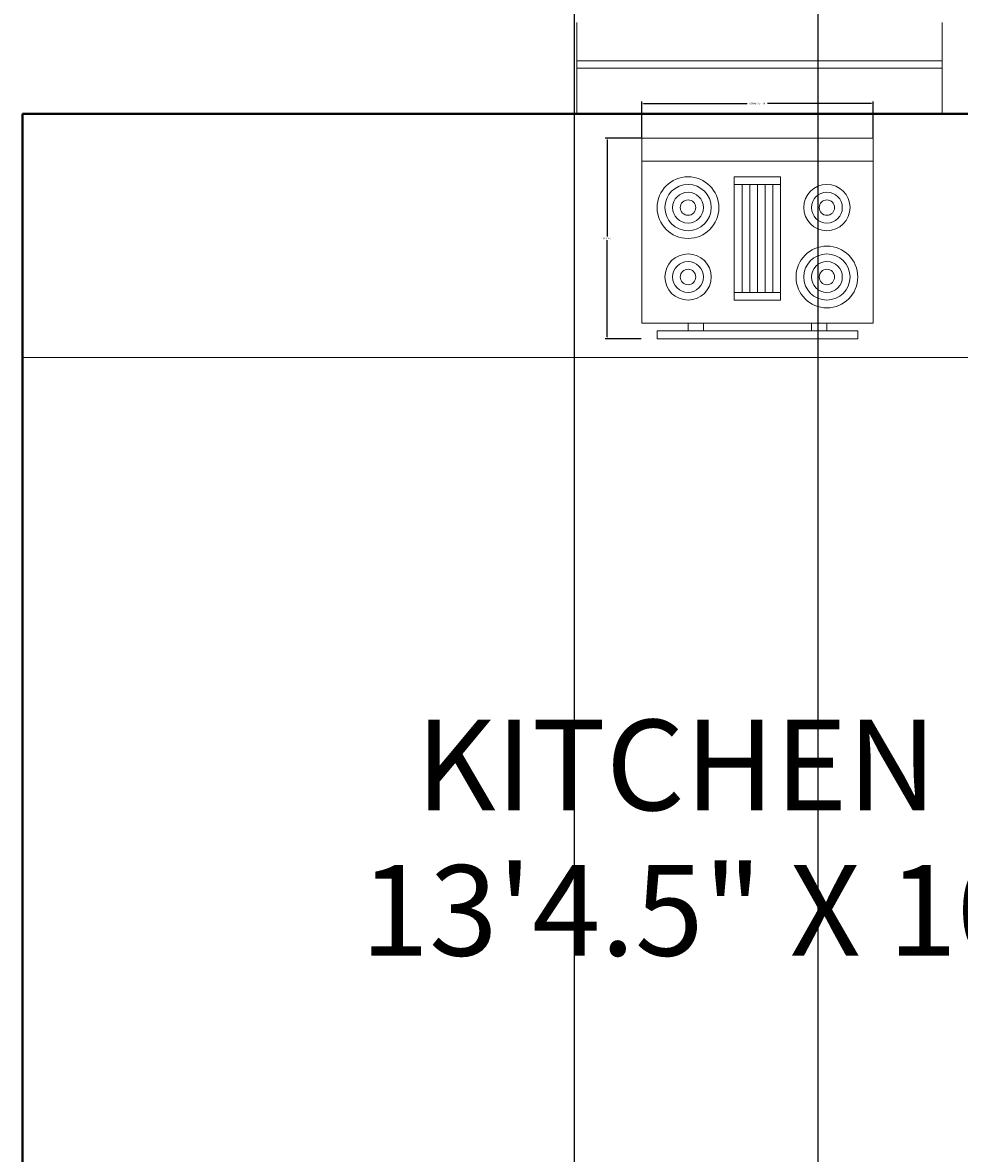
# Model space of a CAD drawing. Units: inches. Extents: x -46 to 1145, y -527 to 760.
# Tile 51 of 57: x 340 to 432, y 548 to 660. Entities that reach past the tile are written whole.
import ezdxf

# ---------------------------------------------------------------- set-up
doc = ezdxf.new("R2010")
doc.units = ezdxf.units.IN
doc.header["$MEASUREMENT"] = 0
for name, color, linetype, lineweight in [('A-ANNO-DIMS', 2, 'Continuous', 18), ('A-AREA-IDEN', 1, 'Continuous', 18), ('A-EQPM', 2, 'Continuous', 18), ('A-FLOR-CASE', 32, 'Continuous', 18), ('WALLS', 4, 'Continuous', 40), ('WINDOWS', 240, 'Continuous', 20)]:
    doc.layers.add(name, color=color, linetype=linetype, lineweight=lineweight)
doc.styles.get("Standard").update_dxf_attribs({"font": 'arial.ttf'})
doc.dimstyles.get("Standard").update_dxf_attribs({"dimtxt": 0.18, "dimasz": 0.18, "dimexe": 0.18, "dimexo": 0.0625, "dimgap": 0.09, "dimtad": 0, "dimtih": 1, "dimtoh": 1, "dimdec": 0, "dimzin": 0, "dimdsep": 46, "dimlunit": 3, "dimtxsty": 'Standard', "dimcen": 0.09, "dimadec": 0, "dimazin": 0, "dimtfac": 1, "dimtdec": 0, "dimtofl": 0, "dimtmove": 0, "dimatfit": 3, "dimfxl": 1, "dimtolj": 1, "dimtzin": 0, "dimarcsym": 0})

# ---------------------------------------------------------------- blocks, each defined once
blk = doc.blocks.new('Range-Oven - 30 in top')
for p, q in [((0, -3), (30, -3)), ((12, -6), (18, -6)), ((13, -20), (13, -6)), ((14, -6), (14, -20)), ((15, -20), (15, -6)), ((16, -6), (16, -20)), ((17, -20), (17, -6)), ((18, -20), (12, -20)), ((6, -24), (6, -25)), ((8, -25), (8, -24)), ((22, -25), (22, -24)), ((24, -24), (24, -25))]:
    blk.add_line(p, q)
for points in [[(0, -24), (0, 0), (30, 0), (30, -24)], [(12, -21), (12, -5), (18, -5), (18, -21)], [(2, -26), (2, -25), (28, -25), (28, -26)]]:
    blk.add_lwpolyline(points, close=True)
for centre, radius in [((6, -9), 4), ((6, -9), 3), ((6, -9), 2), ((24, -9), 3), ((24, -9), 2), ((6, -9), 1), ((24, -9), 1), ((24, -18), 4), ((6, -18), 3), ((6, -18), 2), ((24, -18), 3), ((24, -18), 2), ((6, -18), 1), ((24, -18), 1)]:
    blk.add_circle(centre, radius)
blk = doc.blocks.new('WINDOW-36IN')
for p, q in [((0, 4.5), (0, 9)), ((0, 9), (0, 0)), ((36, 9), (36, 0)), ((0, 5.23), (36, 5.23)), ((0, 4.5), (36, 4.5))]:
    blk.add_line(p, q)
blk = doc.blocks.new('KITCHEN-COUNTER-L')
for p, q in [((136.17, 96), (0, 96)), ((136.17, 24), (136.17, 96)), ((136.17, 0), (136.17, 24))]:
    blk.add_line(p, q)
blk = doc.blocks.new('*D674')
at = {"layer": 'A-ANNO-DIMS', "color": 0, "lineweight": -2, "transparency": 16777216}
for p, q in [((400.56, 648.19), (400.56, 651.73)), ((400.74, 651.55), (410.95, 651.55)), ((423.18, 651.55), (412.96, 651.55)), ((423.36, 648.19), (423.36, 651.73))]:
    blk.add_line(p, q, dxfattribs=at)
at = {"layer": 'A-ANNO-DIMS', "color": 0, "transparency": 16777216}
for points in [[(400.74, 651.58), (400.74, 651.52), (400.56, 651.55)], [(423.18, 651.58), (423.18, 651.52), (423.36, 651.55)]]:
    blk.add_solid(points, dxfattribs=at)
at = {"layer": 'Defpoints', "color": 0, "transparency": 16777216}
for p in [(423.36, 651.55), (400.56, 648.13), (423.36, 648.13)]:
    blk.add_point(p, dxfattribs=at)
at = {"layer": 'A-ANNO-DIMS', "color": 0, "transparency": 16777216, "insert": (411.96, 651.55), "char_height": 0.18, "attachment_point": 5}
blk.add_mtext('\\A1;RANGE 23 TYP.', dxfattribs=at)
blk = doc.blocks.new('*D675')
at = {"layer": 'A-ANNO-DIMS', "color": 0, "lineweight": -2, "transparency": 16777216}
for p, q in [((400.49, 648.13), (396.96, 648.13)), ((397.14, 647.95), (397.14, 638.43)), ((397.14, 628.54), (397.14, 638.06)), ((400.49, 628.36), (396.96, 628.36))]:
    blk.add_line(p, q, dxfattribs=at)
at = {"layer": 'A-ANNO-DIMS', "color": 0, "transparency": 16777216}
for points in [[(397.11, 647.95), (397.17, 647.95), (397.14, 648.13)], [(397.11, 628.54), (397.17, 628.54), (397.14, 628.36)]]:
    blk.add_solid(points, dxfattribs=at)
at = {"layer": 'Defpoints', "color": 0, "transparency": 16777216}
for p in [(397.14, 648.13), (400.56, 648.13), (400.56, 628.36)]:
    blk.add_point(p, dxfattribs=at)
at = {"layer": 'A-ANNO-DIMS', "color": 0, "transparency": 16777216, "insert": (397.14, 638.24), "char_height": 0.18, "attachment_point": 5}
blk.add_mtext('\\A1;20 TYP.', dxfattribs=at)
blk = doc.blocks.new('*D699')
at = {"layer": 'A-ANNO-DIMS', "color": 0, "lineweight": -2, "transparency": 16777216}
for p, q in [((393.93, 530.58), (393.93, 759.67)), ((394.11, 759.49), (405.71, 759.49)), ((417.75, 759.49), (406.15, 759.49)), ((417.93, 530.58), (417.93, 759.67))]:
    blk.add_line(p, q, dxfattribs=at)
at = {"layer": 'A-ANNO-DIMS', "color": 0, "transparency": 16777216}
for points in [[(394.11, 759.52), (394.11, 759.46), (393.93, 759.49)], [(417.75, 759.52), (417.75, 759.46), (417.93, 759.49)]]:
    blk.add_solid(points, dxfattribs=at)
at = {"layer": 'Defpoints', "color": 0, "transparency": 16777216}
for p in [(417.93, 759.49), (393.93, 530.52), (417.93, 530.52)]:
    blk.add_point(p, dxfattribs=at)
at = {"layer": 'A-ANNO-DIMS', "color": 0, "transparency": 16777216, "insert": (405.93, 759.49), "char_height": 0.18, "attachment_point": 5}
blk.add_mtext('\\A1;24', dxfattribs=at)

msp = doc.modelspace()

# ---------------------------------------------------------------- linework, layer by layer
at = {"layer": 'WALLS'}
for q in [(339.5637, 530.5176), (500.0637, 650.5176)]:
    msp.add_line((339.5637, 650.5176), q, dxfattribs=at)

# ---------------------------------------------------------------- block references
at = {"layer": 'A-EQPM', "xscale": 0.7600381531222953, "yscale": 0.7600381531222953, "zscale": 0.7600381531222953}
msp.add_blockref('Range-Oven - 30 in top', (400.5568, 648.1251), dxfattribs=at)
at = {"layer": 'A-FLOR-CASE'}
msp.add_blockref('KITCHEN-COUNTER-L', (339.564, 530.518), dxfattribs=at)
at = {"layer": 'WINDOWS'}
msp.add_blockref('WINDOW-36IN', (394.1543, 650.518), dxfattribs=at)

# ---------------------------------------------------------------- texts
at = {"layer": 'A-AREA-IDEN'}
for s, height, p in [('  KITCHEN', 8.92326, (372.8531, 581.8845)), ('13\'4.5" X 10\'0"', 8.923264, (372.8531, 567.5501))]:
    msp.add_text(s, height=height, dxfattribs=at).set_placement(p)

# ---------------------------------------------------------------- dimensions: what is measured, and where the dimension line sits
at = {"layer": 'A-ANNO-DIMS'}
dim = msp.add_linear_dim(base=(417.9282, 759.4886), p1=(393.9282, 530.5176), p2=(417.9282, 530.5176), dimstyle='Standard', override={"dimdec": 0, "dimlfac": 1, "dimrnd": 0, "dimzin": 0, "dimdsep": 46, "dimlunit": 2}, dxfattribs=at)
dim.commit()
dim.dimension.update_dxf_attribs({"geometry": '*D699', "text_midpoint": (405.9282, 759.4886)})
dim = msp.add_linear_dim(base=(423.358, 651.5453), p1=(400.5568, 648.1251), p2=(423.358, 648.1251), text='RANGE <> TYP.', dimstyle='Standard', override={"dimdec": 0, "dimlfac": 1, "dimrnd": 0, "dimzin": 0, "dimdsep": 46, "dimlunit": 2}, dxfattribs=at)
dim.commit()
dim.dimension.update_dxf_attribs({"geometry": '*D674', "text_midpoint": (411.9574, 651.5453)})
dim = msp.add_linear_dim(base=(397.1367, 648.1251), p1=(400.5568, 628.3642), p2=(400.5568, 648.1251), angle=90, text='<> TYP.', dimstyle='Standard', override={"dimdec": 0, "dimlfac": 1, "dimrnd": 0, "dimzin": 0, "dimdsep": 46, "dimlunit": 2}, dxfattribs=at)
dim.commit()
dim.dimension.update_dxf_attribs({"geometry": '*D675', "text_midpoint": (397.1367, 638.2447)})

doc.saveas('drawing.dxf')
